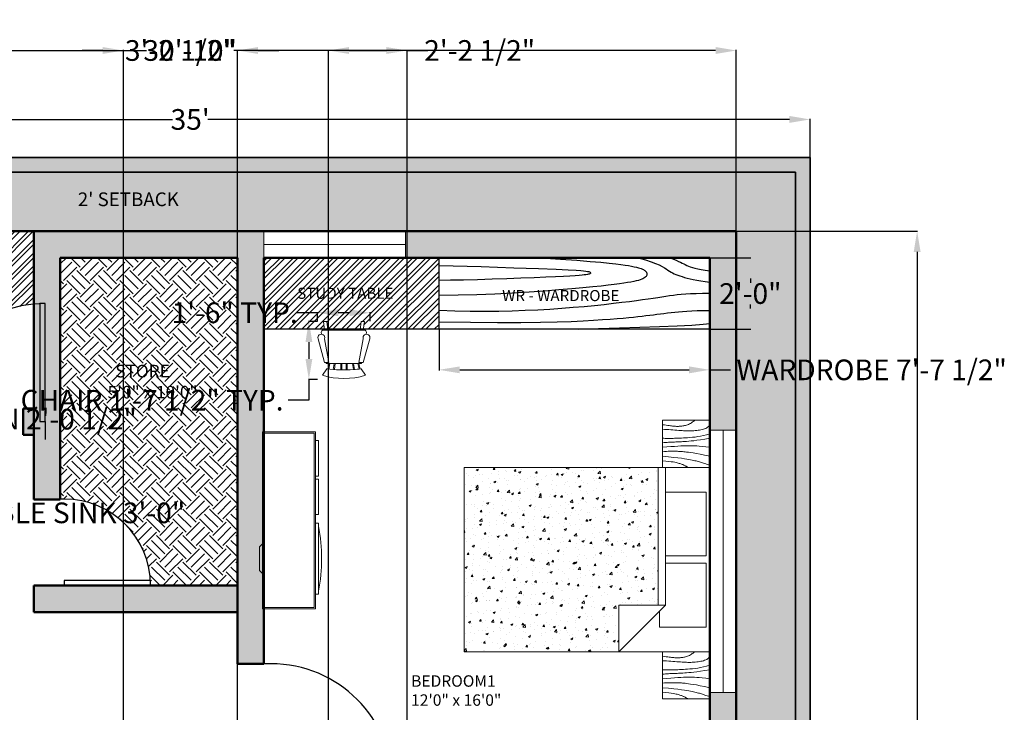
# Model space of a CAD drawing. Units: inches. Extents: x 319 to 870, y 210 to 995.
# Tile 6 of 6: x 524 to 857, y 761 to 995. Entities that reach past the tile are written whole.
import ezdxf

# ---------------------------------------------------------------- set-up
doc = ezdxf.new("R2010")
doc.units = ezdxf.units.IN
doc.header["$MEASUREMENT"] = 0
for name, color, linetype, lineweight in [('A-ANNO-DIMS', 2, 'Continuous', 18), ('A-ANNO-TEXT', 7, 'Continuous', 18), ('A-AREA-IDEN', 7, 'Continuous', 18), ('A-DOOR', 4, 'Continuous', 25), ('A-FLOR-CASE', 7, 'Continuous', 25), ('A-FLOR-CASE-PATT', 252, 'Continuous', 13), ('A-FLOR-PATT', 252, 'Continuous', 13), ('A-FURN', 8, 'Continuous', 18), ('A-GLAZ', 4, 'Continuous', 18), ('A-WALL', 7, 'Continuous', 50), ('A-WALL-PATT', 8, 'Continuous', 13), ('C-PROP', 7, 'Continuous', 35), ('C-PROP-PATT', 8, 'Continuous', 13)]:
    doc.layers.add(name, color=color, linetype=linetype, lineweight=lineweight)
doc.layers.add('A-FURN-PATT', color=30, linetype='Continuous', lineweight=13, true_color=0xf7941d)
doc.layers.add('C-SITE-PATT', color=126, linetype='Continuous', lineweight=13, true_color=0x1e6f63)
doc.styles.get("Standard").update_dxf_attribs({"font": 'arial.ttf'})
doc.dimstyles.get("Standard").update_dxf_attribs({"dimtxt": 7, "dimasz": 7, "dimexe": 0.18, "dimexo": 0.0625, "dimgap": 0.09, "dimtad": 0, "dimtih": 1, "dimtoh": 1, "dimdec": 0, "dimzin": 0, "dimdsep": 46, "dimlunit": 3, "dimtxsty": 'Standard', "dimcen": 0.09, "dimadec": 0, "dimazin": 0, "dimtfac": 1, "dimtdec": 0, "dimtofl": 0, "dimtmove": 0, "dimatfit": 3, "dimfxl": 1, "dimtolj": 1, "dimtzin": 0, "dimarcsym": 0})
pattern_1 = [(45, (0, 0), (-2.245064, 2.245064), []), (45, (0, 1.5875), (-2.245064, 2.245064), [])]

# ---------------------------------------------------------------- blocks, each defined once
blk = doc.blocks.new('Bed - Queen')
for p, q in [((0, -80.00003), (0, 0)), ((0, 0), (59.99999, 0)), ((59.99999, 0), (59.99999, -80.00003)), ((7.99999, -1.2), (28.79998, -1.2)), ((7.99999, -14.4), (7.99999, -1.2)), ((28.79998, -1.2), (28.79998, -14.4)), ((31.19999, -1.2), (51.99999, -1.2)), ((31.19999, -14.4), (31.19999, -1.2)), ((51.99999, -1.2), (51.99999, -16.4)), ((0, -14.4), (44.8, -14.4)), ((59.99999, -29.6), (44.8, -14.4)), ((44.8, -14.4), (44.8, -29.6)), ((44.8, -16.8), (0, -16.8)), ((51.99999, -16.4), (46.79936, -16.4)), ((44.8, -29.6), (59.99999, -29.6)), ((59.99999, -80.00003), (0, -80.00003))]:
    blk.add_line(p, q)
blk = doc.blocks.new('Hutch - 19 x 72 in.')
for p, q in [((0, -19), (0, 0)), ((0, 0), (71.999994, 0)), ((71.999994, 0), (71.999994, -19)), ((71.999994, -19), (0, -19))]:
    blk.add_line(p, q)
for points in [[(26.99999, 0), (32.30411, -0.35238), (36.66731, -0.66276), (40.20336, -0.93603), (43.02603, -1.17708), (45.2491, -1.39079), (46.98632, -1.58203), (48.35147, -1.7557), (49.45833, -1.91667), (50.40388, -2.06917), (51.21809, -2.21484), (51.91414, -2.35465), (52.5052, -2.48958), (53.00447, -2.6206), (53.42512, -2.7487), (53.78035, -2.87484), (54.08333, -3), (54.34537, -3.12516), (54.57031, -3.2513), (54.76008, -3.37939), (54.91666, -3.51042), (55.04198, -3.64534), (55.13801, -3.78516), (55.2067, -3.93083), (55.24999, -4.08333), (55.26904, -4.24316), (55.26171, -4.40885), (55.22509, -4.57845), (55.15624, -4.75), (55.05224, -4.92155), (54.91015, -5.09115), (54.72704, -5.25684), (54.49999, -5.41667), (54.22493, -5.56934), (53.89322, -5.71615), (53.49511, -5.85905), (53.02083, -6), (52.4606, -6.14095), (51.80468, -6.28385), (51.04329, -6.43066), (50.16666, -6.58333), (49.16007, -6.74381), (47.98892, -6.91406), (46.61368, -7.09603), (44.99478, -7.29167), (43.09268, -7.50293), (40.86783, -7.73177), (38.28067, -7.98014), (35.29166, -8.25), (31.87654, -8.54053), (28.07226, -8.83984), (23.93107, -9.1333), (19.5052, -9.40625), (14.84692, -9.64404), (10.00846, -9.83203), (5.04207, -9.95557), (0, -10)], [(52.99999, 0), (54.87133, -0.53955), (56.39257, -1.03516), (57.61205, -1.48975), (58.57812, -1.90625), (59.3391, -2.2876), (59.94335, -2.63672), (60.4392, -2.95654), (60.87499, -3.25), (61.29247, -3.52002), (61.70702, -3.76953), (62.12743, -4.00146), (62.56249, -4.21875), (63.02099, -4.42432), (63.51171, -4.62109), (64.04345, -4.81201), (64.62499, -5), (65.26489, -5.1875), (65.9707, -5.375), (66.74975, -5.5625), (67.60937, -5.75), (68.55688, -5.9375), (69.5996, -6.125), (70.744867, -6.3125), (71.999994, -6.5)], [(61.49999, 0), (62.35961, -0.35254), (63.08007, -0.66406), (63.68627, -0.94043), (64.20312, -1.1875), (64.65551, -1.41113), (65.06835, -1.61719), (65.46655, -1.81152), (65.87499, -2), (66.31762, -2.1875), (66.81445, -2.375), (67.38452, -2.5625), (68.04687, -2.75), (68.82055, -2.9375), (69.7246, -3.125), (70.77807, -3.3125), (71.999994, -3.5)], [(0, -2), (11.2006, -2.34123), (19.90169, -2.62044), (26.43969, -2.84595), (31.15103, -3.02604), (34.37214, -3.16903), (36.43945, -3.2832), (37.68936, -3.37687), (38.45833, -3.45833), (39.02937, -3.53459), (39.472, -3.60742), (39.80232, -3.67733), (40.03645, -3.74479), (40.1905, -3.8103), (40.28059, -3.87435), (40.32283, -3.93742), (40.33333, -4), (40.32405, -4.0625), (40.29036, -4.125), (40.22346, -4.1875), (40.11458, -4.25), (39.95491, -4.3125), (39.73567, -4.375), (39.44807, -4.4375), (39.08333, -4.5), (38.62491, -4.56282), (38.02538, -4.6276), (37.22957, -4.69629), (36.18228, -4.77083), (34.82836, -4.85319), (33.11262, -4.94531), (30.97989, -5.04915), (28.37499, -5.16667), (25.27416, -5.29818), (21.77929, -5.4375), (18.02368, -5.57682), (14.14062, -5.70833), (10.26342, -5.82422), (6.52539, -5.91667), (3.05981, -5.97786), (0, -6)], [(71.999994, -9.5), (70.071934, -9.51147), (68.38801, -9.54492), (66.91113, -9.59888), (65.60416, -9.67187), (64.43001, -9.76245), (63.35156, -9.86914), (62.3317, -9.99048), (61.33333, -10.125), (60.32128, -10.27157), (59.26822, -10.43034), (58.14876, -10.60181), (56.93749, -10.78646), (55.60904, -10.98478), (54.13801, -11.19726), (52.49902, -11.4244), (50.66666, -11.66667), (48.62239, -11.92358), (46.37499, -12.19075), (43.9401, -12.46281), (41.33333, -12.73437), (38.57031, -13.00008), (35.66666, -13.25456), (32.63801, -13.49243), (29.49999, -13.70833), (26.26367, -13.89689), (22.92187, -14.05273), (19.46289, -14.17049), (15.875, -14.24479), (12.14648, -14.27026), (8.26562, -14.24154), (4.2207, -14.15324), (0, -14)], [(0, -17), (8.37556, -17.14274), (15.58268, -17.20443), (21.74194, -17.19775), (26.97395, -17.13542), (31.39933, -17.03011), (35.13866, -16.89453), (38.31257, -16.74137), (41.04166, -16.58333), (43.4322, -16.43083), (45.5332, -16.28516), (47.37931, -16.14534), (49.0052, -16.01042), (50.44555, -15.87939), (51.73502, -15.7513), (52.90828, -15.62516), (53.99999, -15.5), (55.04044, -15.37508), (56.04231, -15.25065), (57.01391, -15.1272), (57.96353, -15.00521), (58.89949, -14.88517), (59.83007, -14.76758), (60.76358, -14.65291), (61.70833, -14.54167), (62.6752, -14.43465), (63.68554, -14.33398), (64.76326, -14.24211), (65.93229, -14.16146), (67.21655, -14.09448), (68.63997, -14.04362), (70.226475, -14.01131), (71.999994, -14)], [(36.99999, -19), (42.40038, -18.8125), (47.95312, -18.625), (53.43554, -18.4375), (58.62499, -18.25), (63.29882, -18.0625), (67.23437, -17.875), (70.208978, -17.6875), (71.999994, -17.5)]]:
    blk.add_lwpolyline(points)
blk = doc.blocks.new('Entertainment Center')
for p, q in [((-4, 0), (-5, -1)), ((4, 0), (-4, 0)), ((5, -1), (4, 0)), ((-17, -19), (-17, -1)), ((-17, -1), (43, -1)), ((-16.5, -18.5), (-16.5, -1.5)), ((-16.5, -1.5), (42.5, -1.5)), ((42.5, -1.5), (42.5, -18.5)), ((43, -1), (43, -19)), ((43, -19), (-17, -19)), ((42.5, -18.5), (-16.5, -18.5)), ((-12, -20), (-12, -19)), ((12, -20), (-12, -20)), ((12, -19), (12, -20)), ((15, -20), (15, -19)), ((27, -20), (15, -20)), ((27, -19), (27, -20)), ((28, -20), (28, -19)), ((40, -20), (28, -20)), ((40, -19), (40, -20))]:
    blk.add_line(p, q)
blk.add_arc((0, 40), 61, 259.6111, 280.3889)
blk = doc.blocks.new('Table - Square Woodgrain 42 x 42 in.')
blk.add_line((0, -42), (42, -42))
for points in [[(0, -4), (1.704, -4.2172), (3.2358, -4.4188), (4.615, -4.604), (5.8615, -4.7721), (6.9951, -4.9224), (8.0357, -5.0541), (9.0031, -5.1667), (9.9171, -5.2594), (10.7951, -5.3316), (11.6445, -5.3836), (12.4702, -5.4157), (13.277, -5.4283), (14.0698, -5.4217), (14.8535, -5.3964), (15.6331, -5.3526), (16.4133, -5.2908), (17.1986, -5.2103), (17.9913, -5.1062), (18.793, -4.9727), (19.6056, -4.8038), (20.4307, -4.5937), (21.2701, -4.3365), (22.1256, -4.0262), (22.9989, -3.6571), (23.888, -3.2272), (24.7756, -2.7516), (25.6408, -2.2491), (26.4624, -1.7387), (27.2195, -1.2395), (27.891, -0.7703), (28.456, -0.3501), (28.8934, 0.002)], [(0, -42), (0, 0), (42, 0), (42, -42)], [(0, -8), (1.8203, -8.1001), (3.6741, -8.2149), (5.5411, -8.3408), (7.4011, -8.4741), (9.2339, -8.6112), (11.0193, -8.7484), (12.7371, -8.8821), (14.3671, -9.0086), (15.8954, -9.1246), (17.3337, -9.2278), (18.6997, -9.3159), (20.0116, -9.387), (21.2871, -9.4389), (22.5442, -9.4696), (23.8008, -9.477), (25.0749, -9.459), (26.3791, -9.4137), (27.7049, -9.3403), (29.0383, -9.2382), (30.3655, -9.1068), (31.6728, -8.9455), (32.9461, -8.7535), (34.1717, -8.5304), (35.3358, -8.2756), (36.4268, -7.9863), (37.443, -7.6521), (38.3849, -7.2603), (39.253, -6.7986), (40.048, -6.2542), (40.7705, -5.6147), (41.421, -4.8674), (42, -4)], [(42, -12), (39.1784, -12.8621), (36.4519, -13.5654), (33.8246, -14.1294), (31.3004, -14.5731), (28.8832, -14.9161), (26.577, -15.1775), (24.3858, -15.3768), (22.3136, -15.5332), (20.3622, -15.6632), (18.5254, -15.7718), (16.7947, -15.8612), (15.1618, -15.9338), (13.6183, -15.9916), (12.1558, -16.0369), (10.7659, -16.0718), (9.4403, -16.0987), (8.1703, -16.1191), (6.9461, -16.1325), (5.7577, -16.1377), (4.595, -16.1335), (3.4479, -16.1188), (2.3064, -16.0924), (1.1604, -16.0532), (0, -16)], [(42, -16), (37.6529, -16.7365), (33.8802, -17.329), (30.6179, -17.7961), (27.8015, -18.1561), (25.3668, -18.4275), (23.2497, -18.6288), (21.3859, -18.7785), (19.7111, -18.8949), (18.1693, -18.9939), (16.7375, -19.0795), (15.401, -19.1534), (14.1449, -19.217), (12.9544, -19.2717), (11.8148, -19.3191), (10.7113, -19.3606), (9.6291, -19.3976), (8.5534, -19.4323), (7.47, -19.4689), (6.3643, -19.5122), (5.222, -19.5672), (4.0288, -19.6386), (2.7703, -19.7313), (1.4321, -19.8501), (0, -20)], [(0, -24), (3.9243, -23.6805), (7.4766, -23.4138), (10.6891, -23.1954), (13.5943, -23.0205), (16.2247, -22.8847), (18.6125, -22.7832), (20.7903, -22.7116), (22.7903, -22.6651), (24.6563, -22.642), (26.4764, -22.6507), (28.35, -22.7024), (30.3766, -22.8084), (32.6555, -22.98), (35.2861, -23.2283), (38.3678, -23.5645), (42, -24)], [(42, -32), (37.392, -31.017), (33.4585, -30.2231), (30.1291, -29.5949), (27.3334, -29.109), (25.0009, -28.742), (23.0612, -28.4707), (21.4439, -28.2716), (20.0786, -28.1215), (18.8998, -28.0002), (17.8609, -27.9014), (16.9206, -27.8219), (16.0371, -27.7588), (15.1691, -27.709), (14.2748, -27.6693), (13.3128, -27.6368), (12.2415, -27.6083), (11.0295, -27.5824), (9.6867, -27.5643), (8.233, -27.5608), (6.6884, -27.5787), (5.0728, -27.6248), (3.4062, -27.7058), (1.7086, -27.8286), (0, -28)], [(0, -32), (5.4026, -32.5358), (9.9494, -33.019), (13.7424, -33.4553), (16.8834, -33.8505), (19.4743, -34.2106), (21.6171, -34.5413), (23.4136, -34.8486), (24.9657, -35.1382), (26.3614, -35.4156), (27.6332, -35.6841), (28.7995, -35.9467), (29.8788, -36.2064), (30.8897, -36.4661), (31.8507, -36.7288), (32.7802, -36.9973), (33.6968, -37.2747), (34.6175, -37.5635), (35.5531, -37.8651), (36.5128, -38.1805), (37.506, -38.5108), (38.5421, -38.8568), (39.6302, -39.2197), (40.7797, -39.6004), (42, -40)], [(0, -36), (3.0098, -36.2857), (5.5354, -36.5643), (7.6368, -36.8359), (9.374, -37.1009), (10.807, -37.3597), (11.9957, -37.6126), (13.0002, -37.8599), (13.8804, -38.102), (14.6874, -38.3393), (15.4365, -38.5729), (16.1338, -38.8041), (16.7858, -39.0341), (17.3987, -39.264), (17.9787, -39.4952), (18.5322, -39.7288), (19.0655, -39.9662), (19.5832, -40.2081), (20.0842, -40.4544), (20.5657, -40.7046), (21.0249, -40.9581), (21.459, -41.2144), (21.8653, -41.4731), (22.2409, -41.7335), (22.5831, -41.9951)]]:
    blk.add_lwpolyline(points)
blk = doc.blocks.new('*U14')
for p, q in [((0, 0), (0, -6)), ((-36, 0), (-36, -6))]:
    blk.add_line(p, q)
blk.add_lwpolyline([(0, 0), (0, 36), (-1.75, 36), (-1.75, 0)], close=True)
blk.add_arc((0, 0), 36, 90, 180)
blk = doc.blocks.new('*U13')
for p, q in [((-30, 0), (-30, -6)), ((0, 0), (0, -6))]:
    blk.add_line(p, q)
blk.add_lwpolyline([(0, 0), (0, 30), (-1.75, 30), (-1.75, 0)], close=True)
blk.add_arc((0, 0), 30, 90, 180)
blk = doc.blocks.new('*U12')
for p, q in [((0, 0), (0, -6)), ((-40, 0), (-40, -6))]:
    blk.add_line(p, q)
blk.add_lwpolyline([(0, 0), (0, 40), (-1.75, 40), (-1.75, 0)], close=True)
blk.add_arc((0, 0), 40, 90, 180)
blk = doc.blocks.new('Chair - Rocking')
for p, q in [((-8, -4.5), (-10, -1.5)), ((-7.5, -4.5), (-7, -7)), ((-6.5, -7), (-7.02225, -4.43)), ((-4.5, -7), (-4.96674, -4.19951)), ((-4, -7), (-4.40532, -4.16272)), ((-1.5, -4.05012), (-1.5, -7)), ((-1, -7), (-1, -4.05012)), ((1, -7), (1, -4.04655)), ((1.5, -4.05012), (1.5, -7)), ((4, -7), (4.40187, -4.18694)), ((4.5, -7), (4.96761, -4.19437)), ((6.5, -7), (7, -4.4057)), ((7.5, -4.5), (7, -7)), ((8, -4.5), (10, -1.5)), ((-9, -7.5), (-12, -18.49999)), ((-7, -7.5), (-9, -7.5)), ((-9, -18.49999), (-7, -7.5)), ((-8.23428, -6.99939), (-8.3093, -7.47958)), ((-8.23041, -7), (8.23915, -7)), ((7, -7.5), (9, -7.5)), ((9, -18.49999), (7, -7.5)), ((8.31071, -7.48854), (8.23449, -7.00073)), ((9, -7.5), (12, -18.49999)), ((-10.36644, -20.64523), (-10.5, -21.49999)), ((-9, -22.49999), (-9.5, -26.49999)), ((0, -22.49999), (-9.5, -22.49999)), ((-8, -26.49999), (-7.5, -22.49999)), ((0, -22.49999), (9.5, -22.49999)), ((8, -26.49999), (7.5, -22.49999)), ((9, -22.49999), (9.5, -26.49999)), ((10.5, -21.49999), (10.3575, -20.58798)), ((-9.5, -26.49999), (-8, -26.49999)), ((9.5, -26.49999), (8, -26.49999))]:
    blk.add_line(p, q)
for centre, radius, start, end in [((0, -34.08333), 34.08333, 72.93847, 107.0615), ((0, -68.25004), 64.25, 93.92211, 97.15267), ((0, -68.25004), 64.25, 82.84733, 93.92211), ((-10.5, -18.99999), 1.58114, 161.5651, 18.43495), ((-9.5, -21.49999), 1, 180, 270), ((10.5, -18.99999), 1.58114, 161.5651, 18.43495), ((9.5, -21.49999), 1, 270, 0)]:
    blk.add_arc(centre, radius, start, end)
blk = doc.blocks.new('*D23')
at = {"layer": 'A-ANNO-DIMS', "color": 0, "lineweight": -2, "transparency": 16777216}
for p, q in [((371.68, 948.73), (371.68, 961.74)), ((378.68, 961.56), (575.66, 961.56)), ((784.68, 961.56), (587.71, 961.56)), ((791.68, 948.73), (791.68, 961.74))]:
    blk.add_line(p, q, dxfattribs=at)
at = {"layer": 'A-ANNO-DIMS', "color": 0, "transparency": 16777216}
for points in [[(378.68, 962.73), (378.68, 960.39), (371.68, 961.56)], [(784.68, 962.73), (784.68, 960.39), (791.68, 961.56)]]:
    blk.add_solid(points, dxfattribs=at)
at = {"layer": 'Defpoints', "color": 0, "transparency": 16777216}
for p in [(791.68, 961.56), (371.68, 948.67), (791.68, 948.67)]:
    blk.add_point(p, dxfattribs=at)
at = {"layer": 'A-ANNO-DIMS', "color": 0, "transparency": 16777216, "insert": (581.68, 961.56), "char_height": 7, "attachment_point": 5}
blk.add_mtext("\\A1;35'", dxfattribs=at)
blk = doc.blocks.new('*D25')
at = {"layer": 'A-ANNO-DIMS', "color": 0, "lineweight": -2, "transparency": 16777216}
for p, q in [((624.79, 893.12), (621.72, 893.12)), ((621.9, 886.12), (621.9, 880.43)), ((624.79, 873.43), (621.72, 873.43)), ((621.9, 873.43), (621.9, 866.43)), ((621.9, 866.43), (614.9, 866.43))]:
    blk.add_line(p, q, dxfattribs=at)
at = {"layer": 'A-ANNO-DIMS', "color": 0, "transparency": 16777216}
for points in [[(620.74, 886.12), (623.07, 886.12), (621.9, 893.12)], [(620.74, 880.43), (623.07, 880.43), (621.9, 873.43)]]:
    blk.add_solid(points, dxfattribs=at)
at = {"layer": 'Defpoints', "color": 0, "transparency": 16777216}
for p in [(624.86, 893.12), (621.9, 873.43), (624.86, 873.43)]:
    blk.add_point(p, dxfattribs=at)
at = {"layer": 'A-ANNO-DIMS', "color": 0, "transparency": 16777216, "insert": (568.79, 866.43), "char_height": 7, "attachment_point": 5}
blk.add_mtext('\\A1;CHAIR 1\'-7 1/2" TYP.', dxfattribs=at)
blk = doc.blocks.new('*D26')
at = {"layer": 'A-ANNO-DIMS', "color": 0, "lineweight": -2, "transparency": 16777216}
for p, q in [((624.86, 896.07), (617.86, 896.07)), ((624.86, 893.18), (624.86, 896.25)), ((635.67, 896.07), (631.86, 896.07)), ((642.67, 893.18), (642.67, 896.25))]:
    blk.add_line(p, q, dxfattribs=at)
at = {"layer": 'A-ANNO-DIMS', "color": 0, "transparency": 16777216}
for points in [[(631.86, 897.24), (631.86, 894.9), (624.86, 896.07)], [(635.67, 897.24), (635.67, 894.9), (642.67, 896.07)]]:
    blk.add_solid(points, dxfattribs=at)
at = {"layer": 'Defpoints', "color": 0, "transparency": 16777216}
for p in [(624.86, 896.07), (624.86, 893.12), (642.67, 893.12)]:
    blk.add_point(p, dxfattribs=at)
at = {"layer": 'A-ANNO-DIMS', "color": 0, "transparency": 16777216, "insert": (596.76, 896.07), "char_height": 7, "attachment_point": 5}
blk.add_mtext('\\A1;1\'-6" TYP.', dxfattribs=at)
blk = doc.blocks.new('*D33')
at = {"layer": 'A-ANNO-DIMS', "color": 0, "lineweight": -2, "transparency": 16777216}
for p, q in [((665.99, 890.41), (665.99, 876.54)), ((757.68, 890.41), (757.68, 876.54)), ((672.99, 876.72), (750.68, 876.72)), ((757.68, 876.72), (764.68, 876.72))]:
    blk.add_line(p, q, dxfattribs=at)
at = {"layer": 'A-ANNO-DIMS', "color": 0, "transparency": 16777216}
for points in [[(672.99, 877.88), (672.99, 875.55), (665.99, 876.72)], [(750.68, 877.88), (750.68, 875.55), (757.68, 876.72)]]:
    blk.add_solid(points, dxfattribs=at)
at = {"layer": 'Defpoints', "color": 0, "transparency": 16777216}
for p in [(665.99, 890.47), (757.68, 890.47), (757.68, 876.72)]:
    blk.add_point(p, dxfattribs=at)
at = {"layer": 'A-ANNO-DIMS', "color": 0, "transparency": 16777216, "insert": (812.53, 876.72), "char_height": 7, "attachment_point": 5}
blk.add_mtext('\\A1;WARDROBE 7\'-7 1/2"', dxfattribs=at)
blk = doc.blocks.new('*D34')
at = {"layer": 'A-ANNO-DIMS', "color": 0, "lineweight": -2, "transparency": 16777216}
for p, q in [((757.75, 914.67), (771.62, 914.67)), ((771.44, 907.67), (771.44, 906.23)), ((771.44, 897.47), (771.44, 898.91)), ((757.75, 890.47), (771.62, 890.47))]:
    blk.add_line(p, q, dxfattribs=at)
at = {"layer": 'A-ANNO-DIMS', "color": 0, "transparency": 16777216}
for points in [[(770.27, 907.67), (772.61, 907.67), (771.44, 914.67)], [(770.27, 897.47), (772.61, 897.47), (771.44, 890.47)]]:
    blk.add_solid(points, dxfattribs=at)
at = {"layer": 'Defpoints', "color": 0, "transparency": 16777216}
for p in [(757.68, 914.67), (771.44, 914.67), (757.68, 890.47)]:
    blk.add_point(p, dxfattribs=at)
at = {"layer": 'A-ANNO-DIMS', "color": 0, "transparency": 16777216, "insert": (771.44, 902.57), "char_height": 7, "attachment_point": 5}
blk.add_mtext('\\A1;2\'-0"', dxfattribs=at)
blk = doc.blocks.new('*D43')
at = {"layer": 'A-ANNO-DIMS', "color": 0, "lineweight": -2, "transparency": 16777216}
for p, q in [((451.25, 833.61), (451.25, 828.09)), ((487.25, 833.61), (487.25, 828.09)), ((458.25, 828.27), (480.25, 828.27)), ((487.25, 828.27), (494.25, 828.27))]:
    blk.add_line(p, q, dxfattribs=at)
at = {"layer": 'A-ANNO-DIMS', "color": 0, "transparency": 16777216}
for points in [[(458.25, 829.44), (458.25, 827.1), (451.25, 828.27)], [(480.25, 829.44), (480.25, 827.1), (487.25, 828.27)]]:
    blk.add_solid(points, dxfattribs=at)
at = {"layer": 'Defpoints', "color": 0, "transparency": 16777216}
for p in [(451.25, 833.67), (487.25, 833.67), (487.25, 828.27)]:
    blk.add_point(p, dxfattribs=at)
at = {"layer": 'A-ANNO-DIMS', "color": 0, "transparency": 16777216, "insert": (537.71, 828.27), "char_height": 7, "attachment_point": 5}
blk.add_mtext('\\A1;DOUBLE SINK 3\'-0"', dxfattribs=at)
blk = doc.blocks.new('*D47')
at = {"layer": 'A-ANNO-DIMS', "color": 0, "lineweight": -2, "transparency": 16777216}
for p, q in [((465.06, 863.63), (465.06, 859.83)), ((489.61, 863.63), (489.61, 859.83)), ((472.06, 860.01), (482.61, 860.01)), ((489.61, 860.01), (496.61, 860.01))]:
    blk.add_line(p, q, dxfattribs=at)
at = {"layer": 'A-ANNO-DIMS', "color": 0, "transparency": 16777216}
for points in [[(472.06, 861.17), (472.06, 858.84), (465.06, 860.01)], [(482.61, 861.17), (482.61, 858.84), (489.61, 860.01)]]:
    blk.add_solid(points, dxfattribs=at)
at = {"layer": 'Defpoints', "color": 0, "transparency": 16777216}
for p in [(465.06, 863.69), (489.61, 863.69), (489.61, 860.01)]:
    blk.add_point(p, dxfattribs=at)
at = {"layer": 'A-ANNO-DIMS', "color": 0, "transparency": 16777216, "insert": (530.04, 860.01), "char_height": 7, "attachment_point": 5}
blk.add_mtext('\\A1;BASIN 2\'-0 1/2"', dxfattribs=at)
blk = doc.blocks.new('*D49')
at = {"layer": 'A-ANNO-DIMS', "color": 0, "lineweight": -2, "transparency": 16777216}
for p, q in [((396.68, 923.73), (396.68, 985.1)), ((403.68, 984.92), (566.85, 984.92)), ((759.68, 984.92), (596.52, 984.92)), ((766.68, 923.73), (766.68, 985.1))]:
    blk.add_line(p, q, dxfattribs=at)
at = {"layer": 'A-ANNO-DIMS', "color": 0, "transparency": 16777216}
for points in [[(403.68, 986.09), (403.68, 983.75), (396.68, 984.92)], [(759.68, 986.09), (759.68, 983.75), (766.68, 984.92)]]:
    blk.add_solid(points, dxfattribs=at)
at = {"layer": 'Defpoints', "color": 0, "transparency": 16777216}
for p in [(766.68, 984.92), (396.68, 923.67), (766.68, 923.67)]:
    blk.add_point(p, dxfattribs=at)
at = {"layer": 'A-ANNO-DIMS', "color": 0, "transparency": 16777216, "insert": (581.68, 984.92), "char_height": 7, "attachment_point": 5}
blk.add_mtext('\\A1;30\'-10"', dxfattribs=at)
blk = doc.blocks.new('*D50')
at = {"layer": 'A-ANNO-DIMS', "color": 0, "lineweight": -2, "transparency": 16777216}
for p, q in [((766.75, 923.67), (828.11, 923.67)), ((827.93, 916.67), (827.93, 669.33)), ((827.93, 414.67), (827.93, 662)), ((757.75, 407.67), (828.11, 407.67))]:
    blk.add_line(p, q, dxfattribs=at)
at = {"layer": 'A-ANNO-DIMS', "color": 0, "transparency": 16777216}
for points in [[(826.77, 916.67), (829.1, 916.67), (827.93, 923.67)], [(826.77, 414.67), (829.1, 414.67), (827.93, 407.67)]]:
    blk.add_solid(points, dxfattribs=at)
at = {"layer": 'Defpoints', "color": 0, "transparency": 16777216}
for p in [(766.68, 923.67), (827.93, 923.67), (757.68, 407.67)]:
    blk.add_point(p, dxfattribs=at)
at = {"layer": 'A-ANNO-DIMS', "color": 0, "transparency": 16777216, "insert": (827.93, 665.67), "char_height": 7, "attachment_point": 5}
blk.add_mtext('\\A1;43\'-0"', dxfattribs=at)
blk = doc.blocks.new('*D55')
at = {"layer": 'A-ANNO-DIMS', "color": 0, "lineweight": -2, "transparency": 16777216}
for p, q in [((628.53, 485.73), (628.53, 985.1)), ((635.53, 984.92), (648.14, 984.92)), ((655.14, 485.73), (655.14, 985.1)), ((655.14, 984.92), (662.14, 984.92))]:
    blk.add_line(p, q, dxfattribs=at)
at = {"layer": 'A-ANNO-DIMS', "color": 0, "transparency": 16777216}
for points in [[(635.53, 986.09), (635.53, 983.75), (628.53, 984.92)], [(648.14, 986.09), (648.14, 983.75), (655.14, 984.92)]]:
    blk.add_solid(points, dxfattribs=at)
at = {"layer": 'Defpoints', "color": 0, "transparency": 16777216}
for p in [(655.14, 984.92), (628.53, 485.67), (655.14, 485.67)]:
    blk.add_point(p, dxfattribs=at)
at = {"layer": 'A-ANNO-DIMS', "color": 0, "transparency": 16777216, "insert": (679.75, 984.92), "char_height": 7, "attachment_point": 5}
blk.add_mtext('\\A1;2\'-2 1/2"', dxfattribs=at)
blk = doc.blocks.new('*D59')
at = {"layer": 'A-ANNO-DIMS', "color": 0, "lineweight": -2, "transparency": 16777216}
for p, q in [((552.06, 984.92), (545.06, 984.92)), ((559.06, 725.73), (559.06, 985.1)), ((597.68, 735.92), (597.68, 985.1)), ((604.68, 984.92), (611.68, 984.92))]:
    blk.add_line(p, q, dxfattribs=at)
at = {"layer": 'A-ANNO-DIMS', "color": 0, "transparency": 16777216}
for points in [[(552.06, 986.09), (552.06, 983.75), (559.06, 984.92)], [(604.68, 986.09), (604.68, 983.75), (597.68, 984.92)]]:
    blk.add_solid(points, dxfattribs=at)
at = {"layer": 'Defpoints', "color": 0, "transparency": 16777216}
for p in [(597.68, 984.92), (597.68, 735.86), (559.06, 725.67)]:
    blk.add_point(p, dxfattribs=at)
at = {"layer": 'A-ANNO-DIMS', "color": 0, "transparency": 16777216, "insert": (578.37, 984.92), "char_height": 7, "attachment_point": 5}
blk.add_mtext('\\A1;3\'-2 1/2"', dxfattribs=at)

msp = doc.modelspace()

# ---------------------------------------------------------------- hatches: boundary and pattern name
at = {"layer": 'A-FLOR-CASE-PATT'}
h = msp.add_hatch(dxfattribs=at)
h.set_pattern_fill('STEEL', color=256)
h.set_pattern_definition(pattern_1)
h.paths.add_polyline_path([(627.17, 890.47), (626.84, 893.12), (627.93, 893.12), (628.26, 890.47), (639.27, 890.47), (639.6, 893.12), (640.69, 893.12), (640.36, 890.47), (665.99, 890.47), (665.99, 914.67), (606.68, 914.67), (606.68, 890.47)])
h.paths.add_polyline_path([(616.77, 898.66), (654.56, 898.66), (654.56, 906.41), (616.77, 906.41)], flags=24)
at = {"layer": 'A-FLOR-PATT'}
h = msp.add_hatch(dxfattribs=at)
h.set_pattern_fill('STEEL', color=256)
h.set_pattern_definition(pattern_1)
h.paths.add_polyline_path([(472.85, 883.14, -0.08192), (477.66, 883.77, -0.08192), (482.42, 882.83, -0.090016), (486.22, 880.56, -0.104469), (488.8, 877.12, -0.117634), (489.57, 873.36, -0.117634), (488.56, 869.67, -0.104469), (485.76, 866.4, -0.090016), (481.83, 864.38, -0.073818), (477.49, 863.73), (492.56, 863.67), (492.82, 863.67, -0.354003), (528.68, 898.98), (528.68, 923.67), (396.68, 923.67), (396.68, 863.67), (404.28, 863.67), (404.28, 893.49), (406.44, 893.49, -1.658066), (407.33, 893.49), (424.73, 893.49, -1.757253), (425.6, 893.49), (427.85, 893.49), (427.85, 863.67), (428.98, 863.67), (428.98, 893.49), (431.02, 893.49, -1.575486), (431.93, 893.49), (450.07, 893.49, -1.717768), (450.95, 893.49), (452.54, 893.49), (452.54, 863.67), (477.49, 863.73, -0.008053), (477.01, 863.74, -0.08192), (472.25, 864.69, -0.090016), (468.46, 866.95, -0.104469), (465.87, 870.4, -0.117634), (465.1, 874.15, -0.117634), (466.11, 877.85, -0.104469), (468.92, 881.12, -0.090016)])
h.paths.add_polyline_path([(475.31, 895.58), (505.85, 895.58), (505.85, 911.01), (475.31, 911.01)], flags=24)
h = msp.add_hatch(dxfattribs=at)
h.set_pattern_fill('EARTH', color=256, angle=45)
h.set_pattern_definition([(45, (0, 0), (0, 8.980256), [6.35, -6.35]), (45, (-1.684, 1.684), (0, 8.980256), [6.35, -6.35]), (45, (-3.3676, 3.3676), (0, 8.980256), [6.35, -6.35]), (135, (-3.3676, 4.49), (-8.980256, 0), [6.35, -6.35]), (135, (-1.684, 6.174), (-8.980256, 0), [6.35, -6.35]), (135, (0, 7.858), (-8.980256, 0), [6.35, -6.35])])
h.paths.add_polyline_path([(597.68, 914.67), (537.68, 914.67), (537.68, 832.93), (539.04, 832.93, -0.39722), (568.25, 805.38), (568.3, 805.38), (568.3, 803.67), (597.68, 803.67)])
h.paths.add_polyline_path([(552.4, 864.59), (583.99, 864.59), (583.99, 880.55), (552.4, 880.55)], flags=24)
at = {"layer": 'A-FURN-PATT'}
h = msp.add_hatch(dxfattribs=at)
h.set_pattern_fill('AR-CONC', color=256)
h.set_pattern_definition([(50, (0, 0), (7.172602, -0.62752), [0.75, -8.25]), (355, (0, 0), (-1.387513, 7.52192), [0.6, -6.6]), (100.45144, (0.598, -0.052), (5.78509, 6.8944), [0.6374, -7.01142]), (46.1842, (0, 2), (10.67241, -1.65519), [1.125, -12.375]), (96.6356, (0.889, 1.862), (9.34662, 9.74119), [0.9561, -10.51714]), (351.1842, (0, 2), (9.34662, 9.74119), [0.9, -9.9]), (21, (1, 1.5), (5.96907, -4.02619), [0.75, -8.25]), (326, (1, 1.5), (2.433153, 7.2515), [0.6, -6.6]), (71.45144, (1.4974, 1.1645), (8.402224, 3.22531), [0.6374, -7.01142]), (37.5, (0, 0), (0.1215986, 3.3289385), [0, -6.52, 0, -6.7, 0, -6.625]), (7.5, (0, 0), (2.630695, 3.944117), [0, -3.82, 0, -6.37, 0, -2.525]), (327.5, (-2.23, 0), (5.3382244, -0.225549), [0, -2.5, 0, -7.8, 0, -10.35]), (317.5, (-3.23, 0), (5.831862, 1.00105), [0, -3.25, 0, -5.18, 0, -7.35])])
h.paths.add_polyline_path([(726.89, 797.03), (740.21, 797.03), (740.21, 843.65), (674.45, 843.65), (674.45, 781.22), (726.89, 781.22)])
at = {"layer": 'A-WALL-PATT'}
h = msp.add_hatch(color=256, dxfattribs=at)
h.dxf.hatch_style = 1
h.paths.add_polyline_path([(528.68, 923.67), (528.68, 832.82), (537.68, 832.82), (537.68, 914.67), (597.68, 914.67), (597.68, 777.1), (606.68, 777.1), (606.68, 914.67), (606.68, 923.67)])
h = msp.add_hatch(color=256, dxfattribs=at)
h.dxf.hatch_style = 1
h.paths.add_polyline_path([(654.58, 923.67), (654.58, 914.67), (757.68, 914.67), (757.68, 856.31), (766.68, 856.31), (766.68, 923.67)])
h = msp.add_hatch(color=256, dxfattribs=at)
h.dxf.hatch_style = 1
h.paths.add_polyline_path([(528.68, 863.67), (525.13, 863.67), (525.13, 854.67), (528.68, 854.67)])
h = msp.add_hatch(color=256, dxfattribs=at)
h.dxf.hatch_style = 1
h.paths.add_polyline_path([(597.68, 794.67), (597.68, 803.67), (537.68, 803.67), (528.68, 803.67), (528.68, 794.67)])
h = msp.add_hatch(color=256, dxfattribs=at)
h.dxf.hatch_style = 1
h.paths.add_polyline_path([(766.68, 731.67), (766.68, 767.38), (757.68, 767.38), (757.68, 731.67), (654.3, 731.67), (654.3, 722.67), (757.68, 722.67), (757.68, 704.22), (766.68, 704.22)])
at = {"layer": 'C-PROP-PATT'}
h = msp.add_hatch(color=256, dxfattribs=at)
h.dxf.hatch_style = 1
h.paths.add_polyline_path([(757.68, 329.67), (597.68, 329.67), (597.68, 324.67), (791.68, 324.67), (791.68, 948.67), (376.68, 948.67), (376.68, 943.67), (786.68, 943.67), (786.68, 329.67), (766.68, 329.67), (766.68, 354.04), (757.68, 354.04)])
at = {"layer": 'C-SITE-PATT'}
h = msp.add_hatch(color=256, dxfattribs=at)
h.dxf.hatch_style = 1
h.paths.add_polyline_path([(376.68, 515.67), (396.68, 515.67), (396.68, 923.67), (528.68, 923.67), (606.68, 923.67), (766.68, 923.67), (766.68, 329.67), (786.68, 329.67), (786.68, 943.67), (376.68, 943.67)])
h.paths.add_polyline_path([(392.17, 638.98), (392.17, 682.3), (381.61, 682.3), (381.61, 638.98)], flags=24)
h.paths.add_polyline_path([(772.77, 716.95), (772.77, 673.64), (783.33, 673.64), (783.33, 716.95)], flags=24)
h.paths.add_polyline_path([(542.27, 929.56), (581.61, 929.56), (581.61, 939.15), (542.27, 939.15)], flags=24)

# ---------------------------------------------------------------- linework, layer by layer
at = {"layer": 'A-FLOR-CASE'}
msp.add_line((665.99, 890.47), (606.68, 890.47), dxfattribs=at)
at = {"layer": 'A-GLAZ'}
for p, q in [((606.68, 914.67), (606.68, 923.67)), ((654.58, 923.67), (654.58, 914.67)), ((606.68, 919.17), (654.58, 919.17)), ((757.68, 856.31), (766.68, 856.31)), ((762.18, 856.31), (762.18, 767.38)), ((766.68, 767.38), (757.68, 767.38))]:
    msp.add_line(p, q, dxfattribs=at)
at = {"layer": 'A-WALL'}
for p, q in [((528.68, 923.67), (396.68, 923.67)), ((528.68, 923.67), (528.68, 832.82)), ((606.68, 923.67), (528.68, 923.67)), ((766.68, 923.67), (606.68, 923.67)), ((766.68, 329.67), (766.68, 923.67)), ((537.68, 914.67), (537.68, 832.82)), ((597.68, 914.67), (537.68, 914.67)), ((597.68, 914.67), (597.68, 777.1)), ((606.68, 914.67), (606.68, 777.1)), ((757.68, 914.67), (606.68, 914.67)), ((757.68, 914.67), (757.68, 731.67)), ((528.68, 863.67), (525.13, 863.67)), ((525.13, 863.67), (525.13, 854.67)), ((528.68, 854.67), (525.13, 854.67)), ((528.68, 854.67), (528.68, 832.82)), ((528.68, 832.82), (537.68, 832.82)), ((537.68, 803.67), (528.68, 803.67)), ((528.68, 803.67), (528.68, 794.67)), ((528.68, 803.67), (528.68, 794.67)), ((597.68, 803.67), (537.68, 803.67)), ((597.68, 794.67), (528.68, 794.67)), ((606.68, 777.1), (597.68, 777.1))]:
    msp.add_line(p, q, dxfattribs=at)
at = {"layer": 'C-PROP'}
for p, q in [((791.68, 948.67), (371.68, 948.67)), ((791.68, 324.67), (791.68, 948.67)), ((786.68, 943.67), (376.68, 943.67)), ((786.68, 329.67), (786.68, 943.67))]:
    msp.add_line(p, q, dxfattribs=at)

# ---------------------------------------------------------------- block references
at = {"layer": 'A-DOOR'}
msp.add_blockref('*U12', (532.56, 859.17), dxfattribs=at)
at = {"layer": 'A-DOOR', "rotation": 270}
for name, p, xscale, yscale, zscale in [('*U13', (539.04, 803.67), 0.9754286713934874, 0.9754286713934874, 0.9754286713934874), ('*U14', (609.07, 735.86), 1.146791488036304, 1.146791488036304, 1.146791488036304)]:
    msp.add_blockref(name, p, dxfattribs=dict(at, xscale=xscale, yscale=yscale, zscale=zscale))
at = {"layer": 'A-FLOR-CASE', "xscale": 1.2735537523755, "yscale": 1.2735537523755, "zscale": 1.2735537523755}
msp.add_blockref('Hutch - 19 x 72 in.', (665.99, 914.67), dxfattribs=at)
at = {"layer": 'A-FURN'}
for name, p, xscale, yscale, zscale, rotation in [('Chair - Rocking', (633.76, 873.79), 0.7291334553679598, 0.7291334553679598, 0.7291334553679598, 180), ('Bed - Queen', (757.68, 843.65), 1.0404319622762, 1.0404319622762, 1.0404319622762, 270)]:
    msp.add_blockref(name, p, dxfattribs=dict(at, xscale=xscale, yscale=yscale, zscale=zscale, rotation=rotation))
at = {"layer": 'A-FURN', "xscale": 0.3809342412266087, "yscale": 0.3809342412266087, "zscale": 0.3809342412266087}
for p in [(741.69, 859.64), (741.69, 781.22)]:
    msp.add_blockref('Table - Square Woodgrain 42 x 42 in.', p, dxfattribs=at)
at = {"layer": 'A-FURN', "rotation": 90}
msp.add_blockref('Entertainment Center', (605.18, 812.73), dxfattribs=at)

# ---------------------------------------------------------------- texts
at = {"layer": 'A-ANNO-TEXT', "attachment_point": 1}
for s, width, gutter_width, insert, char_height in [("2' SETBACK", 60.2718, 23.27, (543.62, 936.83), 4.654), ('STUDY TABLE', 48.7012, 18.8, (617.95, 904.54), 3.7605), ('WR - WARDROBE', 48.7012, 18.8, (687.37, 903.76), 3.7605)]:
    msp.add_mtext_dynamic_manual_height_columns(s, width=width, gutter_width=gutter_width, heights=[0], dxfattribs=dict(at, insert=insert, char_height=char_height))
at = {"layer": 'A-AREA-IDEN', "attachment_point": 1}
for s, width, gutter_width, insert, char_height in [('  STORE\\P5\'0" x 10\'0"', 55.4041, 21.39, (553.72, 878.43), 4.2781), ('BEDROOM1\\P12\'0" x 16\'0"', 50.1839, 19.38, (656.53, 773.23), 3.875)]:
    msp.add_mtext_dynamic_manual_height_columns(s, width=width, gutter_width=gutter_width, heights=[0], dxfattribs=dict(at, insert=insert, char_height=char_height))

# ---------------------------------------------------------------- dimensions: what is measured, and where the dimension line sits
at = {"layer": 'A-ANNO-DIMS'}
for base, p1, p2, override, picture, middle in [((597.68, 984.92), (559.06, 725.67), (597.68, 735.86), {"dimdec": 1, "dimlfac": 1, "dimrnd": 0, "dimzin": 1, "dimdsep": 46, "dimlunit": 4, "dimfrac": 2}, '*D59', (578.37, 984.92)), ((655.14, 984.92), (628.53, 485.67), (655.14, 485.67), {"dimdec": 1, "dimlfac": 1, "dimrnd": 0, "dimzin": 1, "dimdsep": 46, "dimlunit": 4, "dimfrac": 2}, '*D55', (679.75, 984.92)), ((766.68, 984.92), (396.68, 923.67), (766.68, 923.67), {"dimdec": 1, "dimlfac": 1, "dimrnd": 0, "dimzin": 1, "dimdsep": 46, "dimlunit": 4, "dimfrac": 2}, '*D49', (581.68, 984.92)), ((791.68, 961.56), (371.68, 948.67), (791.68, 948.67), {"dimclrd": 0, "dimclre": 0, "dimclrt": 0}, '*D23', (581.68, 961.56))]:
    dim = msp.add_linear_dim(base=base, p1=p1, p2=p2, dimstyle='Standard', override=override, dxfattribs=at)
    dim.commit()
    dim.dimension.update_dxf_attribs({"geometry": picture, "text_midpoint": middle})
for base, p1, p2, picture, middle in [((827.93, 923.67), (757.68, 407.67), (766.68, 923.67), '*D50', (827.93, 665.67)), ((771.44, 914.67), (757.68, 890.47), (757.68, 914.67), '*D34', (771.44, 902.57))]:
    dim = msp.add_linear_dim(base=base, p1=p1, p2=p2, angle=90, dimstyle='Standard', override={"dimdec": 1, "dimlfac": 1, "dimrnd": 0, "dimzin": 1, "dimdsep": 46, "dimlunit": 4, "dimfrac": 2}, dxfattribs=at)
    dim.commit()
    dim.dimension.update_dxf_attribs({"geometry": picture, "text_midpoint": middle})
for base, p1, p2, angle, text, picture, middle in [((624.86, 896.07), (642.67, 893.12), (624.86, 893.12), 180, '<> TYP.', '*D26', (596.76, 896.07)), ((621.9, 873.43), (624.86, 893.12), (624.86, 873.43), 270, 'CHAIR <> TYP.', '*D25', (568.79, 866.43))]:
    dim = msp.add_linear_dim(base=base, p1=p1, p2=p2, angle=angle, text=text, dimstyle='Standard', override={"dimdec": 1, "dimlfac": 1, "dimrnd": 0, "dimzin": 1, "dimdsep": 46, "dimlunit": 4, "dimfrac": 2}, dxfattribs=at)
    dim.commit()
    dim.dimension.update_dxf_attribs({"geometry": picture, "text_midpoint": middle})
for base, p1, p2, text, picture, middle in [((757.68, 876.72), (665.99, 890.47), (757.68, 890.47), 'WARDROBE <>', '*D33', (812.53, 876.72)), ((489.6129, 860.0071), (465.0621, 863.6897), (489.6129, 863.6897), 'BASIN <>', '*D47', (530.0389, 860.0071)), ((487.25, 828.27), (451.25, 833.67), (487.25, 833.67), 'DOUBLE SINK <>', '*D43', (537.71, 828.27))]:
    dim = msp.add_linear_dim(base=base, p1=p1, p2=p2, text=text, dimstyle='Standard', override={"dimdec": 1, "dimlfac": 1, "dimrnd": 0, "dimzin": 1, "dimdsep": 46, "dimlunit": 4, "dimfrac": 2}, dxfattribs=at)
    dim.commit()
    dim.dimension.update_dxf_attribs({"geometry": picture, "text_midpoint": middle})

doc.saveas('drawing.dxf')
